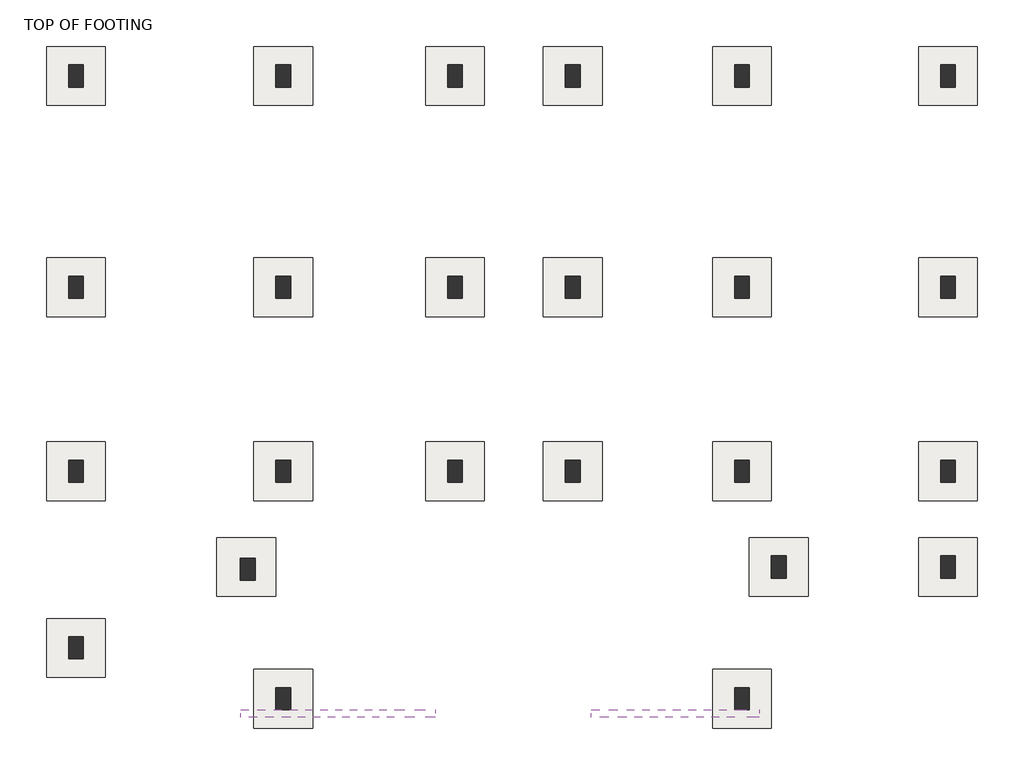
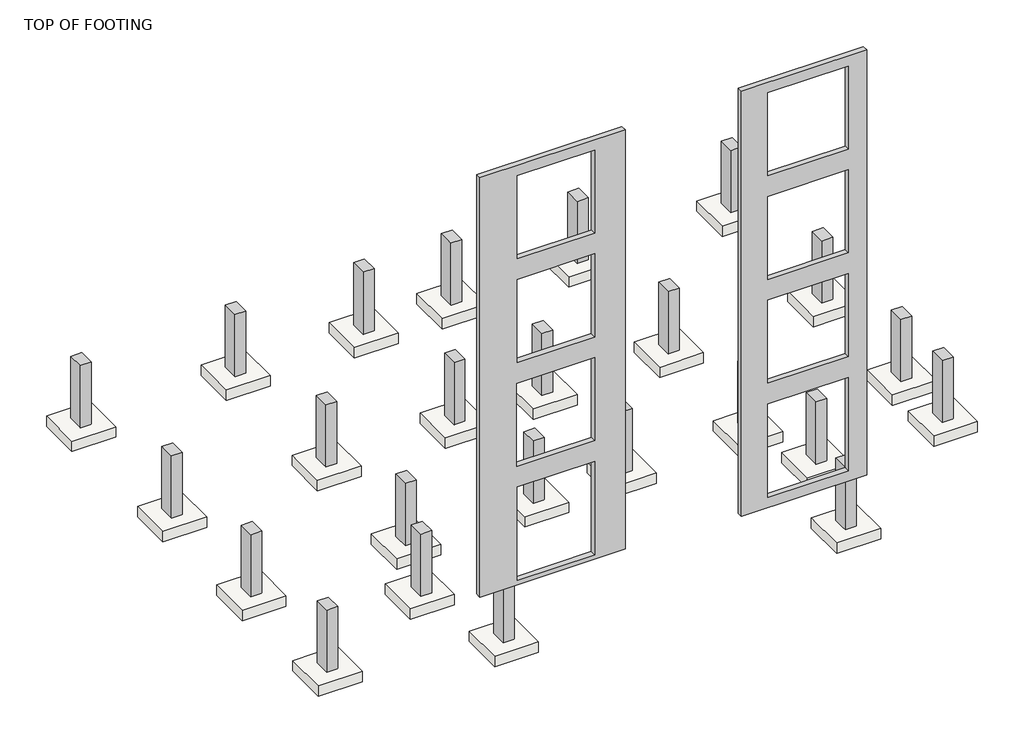
# One storey: 24 columns, 24 slabs, 2 proxies.
"""IFC4 building model written with IfcOpenShell, lengths in millimetres."""

from ifc_helpers import new_model, si_unit, frame, origin, place, context, project, spatial, polyline, outline, extrude, transform, mapped, element, save
from components import generic_models_3_generic_models_3_7d1dbbdc, generic_models_4_generic_models_4_3a94e551, footing_rectangular_4_x_4_x_1_cc6aa31b

model = new_model("IFC4")

# Units and contexts
model_context = context("Model", 3, world=origin())
ifc_project = project(units=[si_unit("LENGTHUNIT", "METRE", prefix="MILLI")], contexts=[model_context])

# Site, building, storey
site = spatial("IfcSite", under=ifc_project)
building = spatial("IfcBuilding", under=site)
storey = spatial("IfcBuildingStorey", under=building, Name="TOP OF FOOTING", Elevation=-1828.8)

# Proxies
placement = place(None, origin())
generic_models_3_generic_models_3_shape = generic_models_3_generic_models_3_7d1dbbdc(model_context)
element("IfcBuildingElementProxy", 1, Name="Generic Models 3 : Generic Models 3", ObjectType="Generic Models 3 : Generic Models 3", at=placement, inside=storey, context=model_context, shape_type="MappedRepresentation", body=[
    mapped(generic_models_3_generic_models_3_shape, transform((0.0, 0.0, 0.0), x_axis=(1.0, 0.0, 0.0), y_axis=(0.0, 1.0, 0.0), z_axis=(0.0, 0.0, 1.0))),
])
generic_models_4_generic_models_4_shape = generic_models_4_generic_models_4_3a94e551(model_context)
element("IfcBuildingElementProxy", 2, Name="Generic Models 4 : Generic Models 4", ObjectType="Generic Models 4 : Generic Models 4", at=placement, inside=storey, context=model_context, shape_type="MappedRepresentation", body=[
    mapped(generic_models_4_generic_models_4_shape, transform((0.0, 0.0, 0.0), x_axis=(1.0, 0.0, 0.0), y_axis=(0.0, 1.0, 0.0), z_axis=(0.0, 0.0, 1.0))),
])

# Columns
element("IfcColumn", 3, ObjectType="Concrete-Rectangular-Column : 1'6\" X 1' COLUMN", at=placement, inside=storey, context=model_context, shape_type="SweptSolid", body=[
    extrude(outline(polyline([(-8839.9786397, -1223.6061634), (-8839.9786397, -1680.8061634), (-9144.7786397, -1680.8061634), (-9144.7786397, -1223.6061634), (-8839.9786397, -1223.6061634)])), frame((0.0, 0.0, -1828.8), z_axis=(0.0, 0.0, 1.0), x_axis=(1.0, 0.0, 0.0)), (0.0, 0.0, 1.0), 1828.8),
])
element("IfcColumn", 4, ObjectType="Concrete-Rectangular-Column : 1'6\" X 1' COLUMN", at=placement, inside=storey, context=model_context, shape_type="SweptSolid", body=[
    extrude(outline(polyline([(-4548.1175798, -1223.6061634), (-4548.1175798, -1680.8061634), (-4852.9175798, -1680.8061634), (-4852.9175798, -1223.6061634), (-4548.1175798, -1223.6061634)])), frame((0.0, 0.0, -1828.8), z_axis=(0.0, 0.0, 1.0), x_axis=(1.0, 0.0, 0.0)), (0.0, 0.0, 1.0), 1828.8),
])
element("IfcColumn", 5, ObjectType="Concrete-Rectangular-Column : 1'6\" X 1' COLUMN", at=placement, inside=storey, context=model_context, shape_type="SweptSolid", body=[
    extrude(outline(polyline([(-992.1175798, -1223.6061634), (-992.1175798, -1680.8061634), (-1296.9175798, -1680.8061634), (-1296.9175798, -1223.6061634), (-992.1175798, -1223.6061634)])), frame((0.0, 0.0, -1828.8), z_axis=(0.0, 0.0, 1.0), x_axis=(1.0, 0.0, 0.0)), (0.0, 0.0, 1.0), 1828.8),
])
element("IfcColumn", 6, ObjectType="Concrete-Rectangular-Column : 1'6\" X 1' COLUMN", at=placement, inside=storey, context=model_context, shape_type="SweptSolid", body=[
    extrude(outline(polyline([(1446.2824202, -1223.6061634), (1446.2824202, -1680.8061634), (1141.4824202, -1680.8061634), (1141.4824202, -1223.6061634), (1446.2824202, -1223.6061634)])), frame((0.0, 0.0, -1828.8), z_axis=(0.0, 0.0, 1.0), x_axis=(1.0, 0.0, 0.0)), (0.0, 0.0, 1.0), 1828.8),
])
element("IfcColumn", 7, ObjectType="Concrete-Rectangular-Column : 1'6\" X 1' COLUMN", at=placement, inside=storey, context=model_context, shape_type="SweptSolid", body=[
    extrude(outline(polyline([(4951.4824202, -1223.6061634), (4951.4824202, -1680.8061634), (4646.6824202, -1680.8061634), (4646.6824202, -1223.6061634), (4951.4824202, -1223.6061634)])), frame((0.0, 0.0, -1828.8), z_axis=(0.0, 0.0, 1.0), x_axis=(1.0, 0.0, 0.0)), (0.0, 0.0, 1.0), 1828.8),
])
element("IfcColumn", 8, ObjectType="Concrete-Rectangular-Column : 1'6\" X 1' COLUMN", at=placement, inside=storey, context=model_context, shape_type="SweptSolid", body=[
    extrude(outline(polyline([(9218.6824202, -1223.6061634), (9218.6824202, -1680.8061634), (8913.8824202, -1680.8061634), (8913.8824202, -1223.6061634), (9218.6824202, -1223.6061634)])), frame((0.0, 0.0, -1828.8), z_axis=(0.0, 0.0, 1.0), x_axis=(1.0, 0.0, 0.0)), (0.0, 0.0, 1.0), 1828.8),
])
element("IfcColumn", 9, ObjectType="Concrete-Rectangular-Column : 1'6\" X 1' COLUMN", at=placement, inside=storey, context=model_context, shape_type="SweptSolid", body=[
    extrude(outline(polyline([(9218.6824202, -5600.6620333), (9218.6824202, -6057.8620333), (8913.8824202, -6057.8620333), (8913.8824202, -5600.6620333), (9218.6824202, -5600.6620333)])), frame((0.0, 0.0, -1828.8), z_axis=(0.0, 0.0, 1.0), x_axis=(1.0, 0.0, 0.0)), (0.0, 0.0, 1.0), 1828.8),
])
element("IfcColumn", 10, ObjectType="Concrete-Rectangular-Column : 1'6\" X 1' COLUMN", at=placement, inside=storey, context=model_context, shape_type="SweptSolid", body=[
    extrude(outline(polyline([(4951.4824202, -5600.6620333), (4951.4824202, -6057.8620333), (4646.6824202, -6057.8620333), (4646.6824202, -5600.6620333), (4951.4824202, -5600.6620333)])), frame((0.0, 0.0, -1828.8), z_axis=(0.0, 0.0, 1.0), x_axis=(1.0, 0.0, 0.0)), (0.0, 0.0, 1.0), 1828.8),
])
element("IfcColumn", 11, ObjectType="Concrete-Rectangular-Column : 1'6\" X 1' COLUMN", at=placement, inside=storey, context=model_context, shape_type="SweptSolid", body=[
    extrude(outline(polyline([(1446.2824202, -5600.6620333), (1446.2824202, -6057.8620333), (1141.4824202, -6057.8620333), (1141.4824202, -5600.6620333), (1446.2824202, -5600.6620333)])), frame((0.0, 0.0, -1828.8), z_axis=(0.0, 0.0, 1.0), x_axis=(1.0, 0.0, 0.0)), (0.0, 0.0, 1.0), 1828.8),
])
element("IfcColumn", 12, ObjectType="Concrete-Rectangular-Column : 1'6\" X 1' COLUMN", at=placement, inside=storey, context=model_context, shape_type="SweptSolid", body=[
    extrude(outline(polyline([(-992.1175798, -5600.6620333), (-992.1175798, -6057.8620333), (-1296.9175798, -6057.8620333), (-1296.9175798, -5600.6620333), (-992.1175798, -5600.6620333)])), frame((0.0, 0.0, -1828.8), z_axis=(0.0, 0.0, 1.0), x_axis=(1.0, 0.0, 0.0)), (0.0, 0.0, 1.0), 1828.8),
])
element("IfcColumn", 13, ObjectType="Concrete-Rectangular-Column : 1'6\" X 1' COLUMN", at=placement, inside=storey, context=model_context, shape_type="SweptSolid", body=[
    extrude(outline(polyline([(-4548.1175798, -5600.6620333), (-4548.1175798, -6057.8620333), (-4852.9175798, -6057.8620333), (-4852.9175798, -5600.6620333), (-4548.1175798, -5600.6620333)])), frame((0.0, 0.0, -1828.8), z_axis=(0.0, 0.0, 1.0), x_axis=(1.0, 0.0, 0.0)), (0.0, 0.0, 1.0), 1828.8),
])
element("IfcColumn", 14, ObjectType="Concrete-Rectangular-Column : 1'6\" X 1' COLUMN", at=placement, inside=storey, context=model_context, shape_type="SweptSolid", body=[
    extrude(outline(polyline([(-8839.9786397, -5600.6620333), (-8839.9786397, -6057.8620333), (-9144.7786397, -6057.8620333), (-9144.7786397, -5600.6620333), (-8839.9786397, -5600.6620333)])), frame((0.0, 0.0, -1828.8), z_axis=(0.0, 0.0, 1.0), x_axis=(1.0, 0.0, 0.0)), (0.0, 0.0, 1.0), 1828.8),
])
element("IfcColumn", 15, ObjectType="Concrete-Rectangular-Column : 1'6\" X 1' COLUMN", at=placement, inside=storey, context=model_context, shape_type="SweptSolid", body=[
    extrude(outline(polyline([(-8839.9786397, -9410.6620333), (-8839.9786397, -9867.8620333), (-9144.7786397, -9867.8620333), (-9144.7786397, -9410.6620333), (-8839.9786397, -9410.6620333)])), frame((0.0, 0.0, -1828.8), z_axis=(0.0, 0.0, 1.0), x_axis=(1.0, 0.0, 0.0)), (0.0, 0.0, 1.0), 1828.8),
])
element("IfcColumn", 16, ObjectType="Concrete-Rectangular-Column : 1'6\" X 1' COLUMN", at=placement, inside=storey, context=model_context, shape_type="SweptSolid", body=[
    extrude(outline(polyline([(-4548.1175798, -9410.6620333), (-4548.1175798, -9867.8620333), (-4852.9175798, -9867.8620333), (-4852.9175798, -9410.6620333), (-4548.1175798, -9410.6620333)])), frame((0.0, 0.0, -1828.8), z_axis=(0.0, 0.0, 1.0), x_axis=(1.0, 0.0, 0.0)), (0.0, 0.0, 1.0), 1828.8),
])
element("IfcColumn", 17, ObjectType="Concrete-Rectangular-Column : 1'6\" X 1' COLUMN", at=placement, inside=storey, context=model_context, shape_type="SweptSolid", body=[
    extrude(outline(polyline([(-992.1175798, -9410.6620333), (-992.1175798, -9867.8620333), (-1296.9175798, -9867.8620333), (-1296.9175798, -9410.6620333), (-992.1175798, -9410.6620333)])), frame((0.0, 0.0, -1828.8), z_axis=(0.0, 0.0, 1.0), x_axis=(1.0, 0.0, 0.0)), (0.0, 0.0, 1.0), 1828.8),
])
element("IfcColumn", 18, ObjectType="Concrete-Rectangular-Column : 1'6\" X 1' COLUMN", at=placement, inside=storey, context=model_context, shape_type="SweptSolid", body=[
    extrude(outline(polyline([(9218.6824202, -11391.8620333), (9218.6824202, -11849.0620333), (8913.8824202, -11849.0620333), (8913.8824202, -11391.8620333), (9218.6824202, -11391.8620333)])), frame((0.0, 0.0, -1828.8), z_axis=(0.0, 0.0, 1.0), x_axis=(1.0, 0.0, 0.0)), (0.0, 0.0, 1.0), 1828.8),
])
element("IfcColumn", 19, ObjectType="Concrete-Rectangular-Column : 1'6\" X 1' COLUMN", at=placement, inside=storey, context=model_context, shape_type="SweptSolid", body=[
    extrude(outline(polyline([(9218.6824202, -9410.6620333), (9218.6824202, -9867.8620333), (8913.8824202, -9867.8620333), (8913.8824202, -9410.6620333), (9218.6824202, -9410.6620333)])), frame((0.0, 0.0, -1828.8), z_axis=(0.0, 0.0, 1.0), x_axis=(1.0, 0.0, 0.0)), (0.0, 0.0, 1.0), 1828.8),
])
element("IfcColumn", 20, ObjectType="Concrete-Rectangular-Column : 1'6\" X 1' COLUMN", at=placement, inside=storey, context=model_context, shape_type="SweptSolid", body=[
    extrude(outline(polyline([(4951.4824202, -9410.6620333), (4951.4824202, -9867.8620333), (4646.6824202, -9867.8620333), (4646.6824202, -9410.6620333), (4951.4824202, -9410.6620333)])), frame((0.0, 0.0, -1828.8), z_axis=(0.0, 0.0, 1.0), x_axis=(1.0, 0.0, 0.0)), (0.0, 0.0, 1.0), 1828.8),
])
element("IfcColumn", 21, ObjectType="Concrete-Rectangular-Column : 1'6\" X 1' COLUMN", at=placement, inside=storey, context=model_context, shape_type="SweptSolid", body=[
    extrude(outline(polyline([(1446.2824202, -9410.6620333), (1446.2824202, -9867.8620333), (1141.4824202, -9867.8620333), (1141.4824202, -9410.6620333), (1446.2824202, -9410.6620333)])), frame((0.0, 0.0, -1828.8), z_axis=(0.0, 0.0, 1.0), x_axis=(1.0, 0.0, 0.0)), (0.0, 0.0, 1.0), 1828.8),
])
element("IfcColumn", 22, ObjectType="Concrete-Rectangular-Column : 1'6\" X 1' COLUMN", at=placement, inside=storey, context=model_context, shape_type="SweptSolid", body=[
    extrude(outline(polyline([(-4548.1175798, -14119.6402089), (-4548.1175798, -14576.8402089), (-4852.9175798, -14576.8402089), (-4852.9175798, -14119.6402089), (-4548.1175798, -14119.6402089)])), frame((0.0, 0.0, -1828.8), z_axis=(0.0, 0.0, 1.0), x_axis=(1.0, 0.0, 0.0)), (0.0, 0.0, 1.0), 1828.8),
])
element("IfcColumn", 23, ObjectType="Concrete-Rectangular-Column : 1'6\" X 1' COLUMN", at=placement, inside=storey, context=model_context, shape_type="SweptSolid", body=[
    extrude(outline(polyline([(-8839.9786397, -13068.2620333), (-8839.9786397, -13525.4620333), (-9144.7786397, -13525.4620333), (-9144.7786397, -13068.2620333), (-8839.9786397, -13068.2620333)])), frame((0.0, 0.0, -1828.8), z_axis=(0.0, 0.0, 1.0), x_axis=(1.0, 0.0, 0.0)), (0.0, 0.0, 1.0), 1828.8),
])
element("IfcColumn", 24, ObjectType="Concrete-Rectangular-Column : 1'6\" X 1' COLUMN", at=placement, inside=storey, context=model_context, shape_type="SweptSolid", body=[
    extrude(outline(polyline([(-5284.7175798, -11442.6620333), (-5284.7175798, -11899.8620333), (-5589.5175798, -11899.8620333), (-5589.5175798, -11442.6620333), (-5284.7175798, -11442.6620333)])), frame((0.0, 0.0, -1828.8), z_axis=(0.0, 0.0, 1.0), x_axis=(1.0, 0.0, 0.0)), (0.0, 0.0, 1.0), 1828.8),
])
element("IfcColumn", 25, ObjectType="Concrete-Rectangular-Column : 1'6\" X 1' COLUMN", at=placement, inside=storey, context=model_context, shape_type="SweptSolid", body=[
    extrude(outline(polyline([(5713.4824202, -11391.8620333), (5713.4824202, -11849.0620333), (5408.6824202, -11849.0620333), (5408.6824202, -11391.8620333), (5713.4824202, -11391.8620333)])), frame((0.0, 0.0, -1828.8), z_axis=(0.0, 0.0, 1.0), x_axis=(1.0, 0.0, 0.0)), (0.0, 0.0, 1.0), 1828.8),
])
element("IfcColumn", 26, ObjectType="Concrete-Rectangular-Column : 1'6\" X 1' COLUMN", at=placement, inside=storey, context=model_context, shape_type="SweptSolid", body=[
    extrude(outline(polyline([(4951.4824202, -14119.6402089), (4951.4824202, -14576.8402089), (4646.6824202, -14576.8402089), (4646.6824202, -14119.6402089), (4951.4824202, -14119.6402089)])), frame((0.0, 0.0, -1828.8), z_axis=(0.0, 0.0, 1.0), x_axis=(1.0, 0.0, 0.0)), (0.0, 0.0, 1.0), 1828.8),
])

# Slabs
element("IfcSlab", 27, ObjectType="Footing-Rectangular : 4' X 4' X 1'", at=placement, inside=storey, context=model_context, shape_type="SweptSolid", body=[
    extrude(outline(polyline([(-8382.7786397, -842.6061634), (-8382.7786397, -2061.8061634), (-9601.9786397, -2061.8061634), (-9601.9786397, -842.6061634), (-8382.7786397, -842.6061634)])), frame((0.0, 0.0, -2133.6), z_axis=(0.0, 0.0, 1.0), x_axis=(1.0, 0.0, 0.0)), (0.0, 0.0, 1.0), 304.8),
])
footing_rectangular_4_x_4_x_1_shape = footing_rectangular_4_x_4_x_1_cc6aa31b(model_context)
element("IfcSlab", 28, ObjectType="Footing-Rectangular : 4' X 4' X 1'", at=placement, inside=storey, context=model_context, shape_type="MappedRepresentation", body=[
    mapped(footing_rectangular_4_x_4_x_1_shape, transform((-4700.5175798, -1452.2061634, -1828.8), x_axis=(1.0, 0.0, 0.0), y_axis=(0.0, 1.0, 0.0), z_axis=(0.0, 0.0, 1.0))),
])
element("IfcSlab", 29, ObjectType="Footing-Rectangular : 4' X 4' X 1'", at=placement, inside=storey, context=model_context, shape_type="MappedRepresentation", body=[
    mapped(footing_rectangular_4_x_4_x_1_shape, transform((-1144.5175798, -1452.2061634, -1828.8), x_axis=(1.0, 0.0, 0.0), y_axis=(0.0, 1.0, 0.0), z_axis=(0.0, 0.0, 1.0))),
])
element("IfcSlab", 30, ObjectType="Footing-Rectangular : 4' X 4' X 1'", at=placement, inside=storey, context=model_context, shape_type="MappedRepresentation", body=[
    mapped(footing_rectangular_4_x_4_x_1_shape, transform((1293.8824202, -1452.2061634, -1828.8), x_axis=(1.0, 0.0, 0.0), y_axis=(0.0, 1.0, 0.0), z_axis=(0.0, 0.0, 1.0))),
])
element("IfcSlab", 31, ObjectType="Footing-Rectangular : 4' X 4' X 1'", at=placement, inside=storey, context=model_context, shape_type="MappedRepresentation", body=[
    mapped(footing_rectangular_4_x_4_x_1_shape, transform((4799.0824202, -1452.2061634, -1828.8), x_axis=(1.0, 0.0, 0.0), y_axis=(0.0, 1.0, 0.0), z_axis=(0.0, 0.0, 1.0))),
])
element("IfcSlab", 32, ObjectType="Footing-Rectangular : 4' X 4' X 1'", at=placement, inside=storey, context=model_context, shape_type="MappedRepresentation", body=[
    mapped(footing_rectangular_4_x_4_x_1_shape, transform((9066.2824202, -1452.2061634, -1828.8), x_axis=(1.0, 0.0, 0.0), y_axis=(0.0, 1.0, 0.0), z_axis=(0.0, 0.0, 1.0))),
])
element("IfcSlab", 33, ObjectType="Footing-Rectangular : 4' X 4' X 1'", at=placement, inside=storey, context=model_context, shape_type="MappedRepresentation", body=[
    mapped(footing_rectangular_4_x_4_x_1_shape, transform((-8992.3786397, -5829.2620333, -1828.8), x_axis=(1.0, 0.0, 0.0), y_axis=(0.0, 1.0, 0.0), z_axis=(0.0, 0.0, 1.0))),
])
element("IfcSlab", 34, ObjectType="Footing-Rectangular : 4' X 4' X 1'", at=placement, inside=storey, context=model_context, shape_type="MappedRepresentation", body=[
    mapped(footing_rectangular_4_x_4_x_1_shape, transform((-8992.3786397, -13296.8620333, -1828.8), x_axis=(1.0, 0.0, 0.0), y_axis=(0.0, 1.0, 0.0), z_axis=(0.0, 0.0, 1.0))),
])
element("IfcSlab", 35, ObjectType="Footing-Rectangular : 4' X 4' X 1'", at=placement, inside=storey, context=model_context, shape_type="MappedRepresentation", body=[
    mapped(footing_rectangular_4_x_4_x_1_shape, transform((9066.2824202, -11620.4620333, -1828.8), x_axis=(1.0, 0.0, 0.0), y_axis=(0.0, 1.0, 0.0), z_axis=(0.0, 0.0, 1.0))),
])
element("IfcSlab", 36, ObjectType="Footing-Rectangular : 4' X 4' X 1'", at=placement, inside=storey, context=model_context, shape_type="MappedRepresentation", body=[
    mapped(footing_rectangular_4_x_4_x_1_shape, transform((9066.2824202, -5829.2620333, -1828.8), x_axis=(1.0, 0.0, 0.0), y_axis=(0.0, 1.0, 0.0), z_axis=(0.0, 0.0, 1.0))),
])
element("IfcSlab", 37, ObjectType="Footing-Rectangular : 4' X 4' X 1'", at=placement, inside=storey, context=model_context, shape_type="MappedRepresentation", body=[
    mapped(footing_rectangular_4_x_4_x_1_shape, transform((-4700.5175798, -5829.2620333, -1828.8), x_axis=(1.0, 0.0, 0.0), y_axis=(0.0, 1.0, 0.0), z_axis=(0.0, 0.0, 1.0))),
])
element("IfcSlab", 38, ObjectType="Footing-Rectangular : 4' X 4' X 1'", at=placement, inside=storey, context=model_context, shape_type="MappedRepresentation", body=[
    mapped(footing_rectangular_4_x_4_x_1_shape, transform((-1144.5175798, -9639.2620333, -1828.8), x_axis=(1.0, 0.0, 0.0), y_axis=(0.0, 1.0, 0.0), z_axis=(0.0, 0.0, 1.0))),
])
element("IfcSlab", 39, ObjectType="Footing-Rectangular : 4' X 4' X 1'", at=placement, inside=storey, context=model_context, shape_type="MappedRepresentation", body=[
    mapped(footing_rectangular_4_x_4_x_1_shape, transform((1293.8824202, -9639.2620333, -1828.8), x_axis=(1.0, 0.0, 0.0), y_axis=(0.0, 1.0, 0.0), z_axis=(0.0, 0.0, 1.0))),
])
element("IfcSlab", 40, ObjectType="Footing-Rectangular : 4' X 4' X 1'", at=placement, inside=storey, context=model_context, shape_type="MappedRepresentation", body=[
    mapped(footing_rectangular_4_x_4_x_1_shape, transform((4799.0824202, -14348.2402089, -1828.8), x_axis=(1.0, 0.0, 0.0), y_axis=(0.0, 1.0, 0.0), z_axis=(0.0, 0.0, 1.0))),
])
element("IfcSlab", 41, ObjectType="Footing-Rectangular : 4' X 4' X 1'", at=placement, inside=storey, context=model_context, shape_type="MappedRepresentation", body=[
    mapped(footing_rectangular_4_x_4_x_1_shape, transform((-4700.5175798, -14348.2402089, -1828.8), x_axis=(1.0, 0.0, 0.0), y_axis=(0.0, 1.0, 0.0), z_axis=(0.0, 0.0, 1.0))),
])
element("IfcSlab", 42, ObjectType="Footing-Rectangular : 4' X 4' X 1'", at=placement, inside=storey, context=model_context, shape_type="MappedRepresentation", body=[
    mapped(footing_rectangular_4_x_4_x_1_shape, transform((4799.0824202, -9639.2620333, -1828.8), x_axis=(1.0, 0.0, 0.0), y_axis=(0.0, 1.0, 0.0), z_axis=(0.0, 0.0, 1.0))),
])
element("IfcSlab", 43, ObjectType="Footing-Rectangular : 4' X 4' X 1'", at=placement, inside=storey, context=model_context, shape_type="MappedRepresentation", body=[
    mapped(footing_rectangular_4_x_4_x_1_shape, transform((4799.0824202, -5829.2620333, -1828.8), x_axis=(1.0, 0.0, 0.0), y_axis=(0.0, 1.0, 0.0), z_axis=(0.0, 0.0, 1.0))),
])
element("IfcSlab", 44, ObjectType="Footing-Rectangular : 4' X 4' X 1'", at=placement, inside=storey, context=model_context, shape_type="MappedRepresentation", body=[
    mapped(footing_rectangular_4_x_4_x_1_shape, transform((1293.8824202, -5829.2620333, -1828.8), x_axis=(1.0, 0.0, 0.0), y_axis=(0.0, 1.0, 0.0), z_axis=(0.0, 0.0, 1.0))),
])
element("IfcSlab", 45, ObjectType="Footing-Rectangular : 4' X 4' X 1'", at=placement, inside=storey, context=model_context, shape_type="MappedRepresentation", body=[
    mapped(footing_rectangular_4_x_4_x_1_shape, transform((-1144.5175798, -5829.2620333, -1828.8), x_axis=(1.0, 0.0, 0.0), y_axis=(0.0, 1.0, 0.0), z_axis=(0.0, 0.0, 1.0))),
])
element("IfcSlab", 46, ObjectType="Footing-Rectangular : 4' X 4' X 1'", at=placement, inside=storey, context=model_context, shape_type="MappedRepresentation", body=[
    mapped(footing_rectangular_4_x_4_x_1_shape, transform((-8992.3786397, -9639.2620333, -1828.8), x_axis=(1.0, 0.0, 0.0), y_axis=(0.0, 1.0, 0.0), z_axis=(0.0, 0.0, 1.0))),
])
element("IfcSlab", 47, ObjectType="Footing-Rectangular : 4' X 4' X 1'", at=placement, inside=storey, context=model_context, shape_type="MappedRepresentation", body=[
    mapped(footing_rectangular_4_x_4_x_1_shape, transform((-4700.5175798, -9639.2620333, -1828.8), x_axis=(1.0, 0.0, 0.0), y_axis=(0.0, 1.0, 0.0), z_axis=(0.0, 0.0, 1.0))),
])
element("IfcSlab", 48, ObjectType="Footing-Rectangular : 4' X 4' X 1'", at=placement, inside=storey, context=model_context, shape_type="MappedRepresentation", body=[
    mapped(footing_rectangular_4_x_4_x_1_shape, transform((9066.2824202, -9639.2620333, -1828.8), x_axis=(1.0, 0.0, 0.0), y_axis=(0.0, 1.0, 0.0), z_axis=(0.0, 0.0, 1.0))),
])
element("IfcSlab", 49, ObjectType="Footing-Rectangular : 4' X 4' X 1'", at=placement, inside=storey, context=model_context, shape_type="MappedRepresentation", body=[
    mapped(footing_rectangular_4_x_4_x_1_shape, transform((5561.0824202, -11620.4620333, -1828.8), x_axis=(1.0, 0.0, 0.0), y_axis=(0.0, 1.0, 0.0), z_axis=(0.0, 0.0, 1.0))),
])
element("IfcSlab", 50, ObjectType="Footing-Rectangular : 4' X 4' X 1'", at=placement, inside=storey, context=model_context, shape_type="MappedRepresentation", body=[
    mapped(footing_rectangular_4_x_4_x_1_shape, transform((-5462.5175798, -11620.4620333, -1828.8), x_axis=(1.0, 0.0, 0.0), y_axis=(0.0, 1.0, 0.0), z_axis=(0.0, 0.0, 1.0))),
])

save(model, "model.ifc")

# Revit data of these elements
# Grids (mm)
#   "1": line (-8992.379, 739.194) -> (-8992.379, -16014.051)
#   "2": line (-4700.518, 739.194) -> (-4700.518, -16014.051)
#   "3": line (-1144.518, -16014.051) -> (-1144.518, 739.194)
#   "4": line (1293.882, -16014.051) -> (1293.882, 739.194)
#   "5": line (4799.082, -16014.051) -> (4799.082, 739.194)
#   "6": line (9066.282, -16014.051) -> (9066.282, 739.194)
#   "A": line (12479.037, -1452.206) -> (-11204.68, -1452.206)
#   "B": line (12479.037, -5829.262) -> (-11204.68, -5829.262)
#   "C": line (12479.037, -9639.262) -> (-11204.68, -9639.262)
#   "D": line (12479.037, -11620.462) -> (-11204.68, -11620.462)
#   "E": line (12479.037, -14348.24) -> (-11204.68, -14348.24)
# Type "Concrete-Rectangular-Column : 1'6\" X 1' COLUMN"
#   Assembly Code = "B10"
#   b = 1' - 0"
#   h = 1' - 6"
#   Structural Material [instance default] = Concrete, Cast-in-Place gray
# Type "Footing-Rectangular : 4' X 4' X 1'"
#   Assembly Code = "A1010100"
#   Width = 4' - 0"
#   Length = 4' - 0"
#   Foundation Thickness = 1' - 0"
#   Structural Material [instance default] = Concrete, Cast-in-Place gray
# Element 1 (IfcBuildingElementProxy, "Generic Models 3 : Generic Models 3")
#   Phase Created = New Construction
#   Materials on its faces: "brown accent frame"
# Element 2 (IfcBuildingElementProxy, "Generic Models 4 : Generic Models 4")
#   Phase Created = New Construction
#   Materials on its faces: "black accent wall"
# Elements 3, 4, 5, 6, 7, 8, 9, 10, 11, 12, 13, 14, 15, 16, 17, 18, 19, 20, 21, 22, 23, 24, 25, 26 (IfcColumn, "Concrete-Rectangular-Column : 1'6\" X 1' COLUMN")
#   Structural Material = WARM BEIGE COLOUR
#   Phase Created = New Construction
#   Materials on its faces: "WARM BEIGE COLOUR"
# Elements 27, 28, 29, 30, 31, 32, 33, 34, 35, 36, 37, 38, 39, 40, 41, 42, 43, 44, 45, 46, 47, 48, 49, 50 (IfcSlab, "Footing-Rectangular : 4' X 4' X 1'")
#   Structural Material = Concrete, Cast-in-Place gray
#   Phase Created = New Construction
#   Materials on its faces: "Concrete, Cast-in-Place gray"
# Materials
#   "Concrete, Cast-in-Place gray": class "Concrete", colour RGB 192 192 192, transparency 0, Description = "Cast-in-place concrete", Cost = 0
#   "brown accent frame": class "Generic", colour RGB 120 120 120, transparency 0, Cost = 0
#   "black accent wall": class "Generic", colour RGB 120 120 120, transparency 0, Cost = 0
#   "WARM BEIGE COLOUR": class "Generic", colour RGB 120 120 120, transparency 0, Cost = 0
